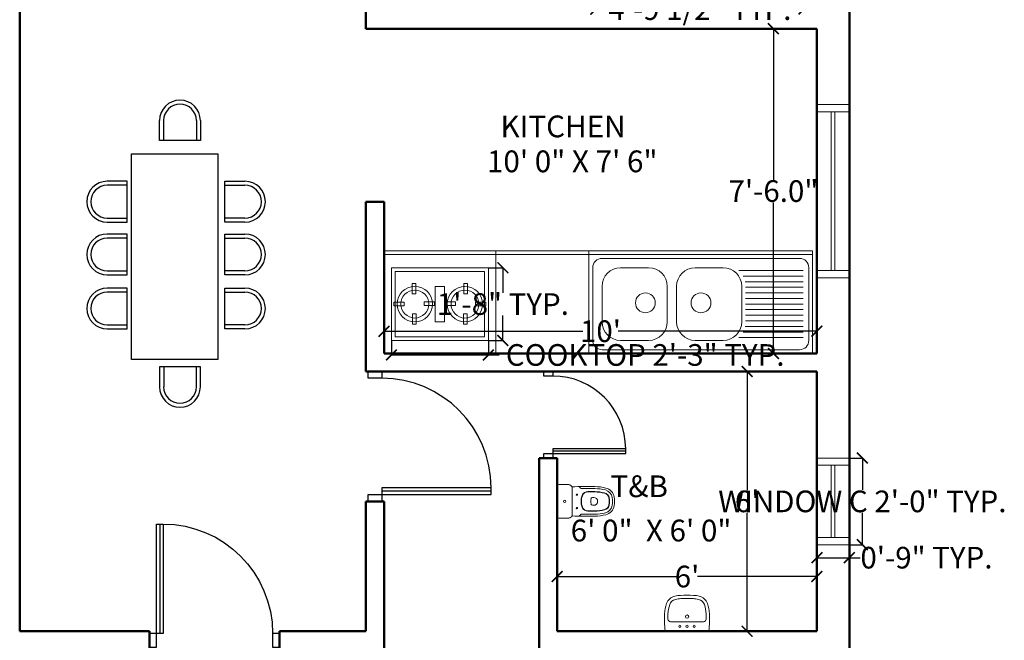
# Model space of a CAD drawing. Units: inches. Extents: x 147 to 1638, y 107 to 941.
# Tile 15 of 17: x 1365 to 1638, y 398 to 570. Entities that reach past the tile are written whole.
import ezdxf

# ---------------------------------------------------------------- set-up
doc = ezdxf.new("R2010")
doc.units = ezdxf.units.IN
doc.header["$MEASUREMENT"] = 0
for name, color, linetype, lineweight in [('A-ANNO-DIMS', 2, 'Continuous', 15), ('A-AREA-IDEN', 7, 'Continuous', 18), ('A-Door', 150, 'Continuous', 25), ('A-EQPM', 8, 'Continuous', 18), ('A-FLOR-CASE', 9, 'Continuous', 20), ('A-FLOR-FIXT', 9, 'Continuous', 18), ('furniture', 50, 'Continuous', 18), ('walls', 7, 'Continuous', 50), ('windows', 3, 'Continuous', 20)]:
    doc.layers.add(name, color=color, linetype=linetype, lineweight=lineweight)
for name, color, linetype in [('A-Glaz', 92, 'Continuous'), ('NT', 1, 'Continuous'), ('家', 40, 'Continuous')]:
    doc.layers.add(name, color=color, linetype=linetype)
doc.styles.get("Standard").update_dxf_attribs({"font": 'arial.ttf'})
doc.dimstyles.get("Standard").update_dxf_attribs({"dimtxt": 6, "dimasz": 3, "dimexe": 0.18, "dimexo": 0.0625, "dimgap": 0.09, "dimtad": 0, "dimtih": 1, "dimtoh": 1, "dimdec": 1, "dimzin": 0, "dimdsep": 46, "dimlunit": 3, "dimtxsty": 'Standard', "dimblk": 'ARCHTICK', "dimcen": 0.09, "dimadec": 0, "dimazin": 0, "dimtfac": 1, "dimtdec": 1, "dimtofl": 0, "dimtmove": 0, "dimatfit": 3, "dimfxl": 1, "dimtolj": 1, "dimtzin": 0, "dimarcsym": 0})

# ---------------------------------------------------------------- blocks, each defined once
blk = doc.blocks.new('A$C087A3AA9')
at = {"layer": 'A-Door'}
for points in [[(852.6, 94.7), (852.6, 852.6), (805.3, 852.6), (805.3, 94.7)], [(47.4, 94.7), (47.4, 0), (0, 0), (0, 94.7)], [(900, 94.7), (900, 0), (852.6, 0), (852.6, 94.7)]]:
    blk.add_lwpolyline(points, close=True, dxfattribs=at)
at = {"layer": 'A-Glaz'}
blk.add_line((828.9, 852.6), (828.9, 94.7), dxfattribs=at)
at = {"layer": 'NT'}
blk.add_arc((805.3, 94.7), 757.9, 90, 180, dxfattribs=at)
blk = doc.blocks.new('_ArchTick')
at = {"color": 0, "linetype": 'ByBlock', "const_width": 0.15}
blk.add_lwpolyline([(-0.5, -0.5), (0.5, 0.5)], dxfattribs=at)
blk = doc.blocks.new('*D40')
at = {"layer": 'A-ANNO-DIMS', "color": 0, "lineweight": -2, "transparency": 16777216}
for p, q in [((1566.2, 472.72), (1566.6, 472.72)), ((1566.42, 472.72), (1566.42, 439.87)), ((1566.42, 400.72), (1566.42, 433.56)), ((1566.2, 400.72), (1566.6, 400.72))]:
    blk.add_line(p, q, dxfattribs=at)
at = {"layer": 'Defpoints', "color": 0, "lineweight": -2, "transparency": 16777216}
for p in [(1566.14, 472.72), (1566.14, 400.72), (1566.42, 400.72)]:
    blk.add_point(p, dxfattribs=at)
at = {"layer": 'A-ANNO-DIMS', "color": 0, "lineweight": -2, "transparency": 16777216, "xscale": 3, "yscale": 3, "zscale": 3}
for p, rotation in [((1566.42, 472.72), 90), ((1566.42, 400.72), 270)]:
    blk.add_blockref('_ArchTick', p, dxfattribs=dict(at, rotation=rotation))
at = {"layer": 'A-ANNO-DIMS', "color": 0, "transparency": 16777216, "insert": (1566.42, 436.72), "char_height": 6, "attachment_point": 5}
blk.add_mtext("\\A1;6'", dxfattribs=at)
blk = doc.blocks.new('*D41')
at = {"layer": 'A-ANNO-DIMS', "color": 0, "lineweight": -2, "transparency": 16777216}
for p, q in [((1513.77, 415.95), (1513.77, 416.07)), ((1513.77, 415.89), (1546.9, 415.89)), ((1585.77, 415.89), (1552.63, 415.89)), ((1585.77, 415.95), (1585.77, 416.07))]:
    blk.add_line(p, q, dxfattribs=at)
at = {"layer": 'Defpoints', "color": 0, "lineweight": -2, "transparency": 16777216}
for p in [(1513.77, 415.89), (1585.77, 415.89), (1585.77, 415.89)]:
    blk.add_point(p, dxfattribs=at)
at = {"layer": 'A-ANNO-DIMS', "color": 0, "lineweight": -2, "transparency": 16777216, "xscale": 3, "yscale": 3, "zscale": 3, "rotation": 180}
blk.add_blockref('_ArchTick', (1513.77, 415.89), dxfattribs=at)
at = {"layer": 'A-ANNO-DIMS', "color": 0, "lineweight": -2, "transparency": 16777216, "xscale": 3, "yscale": 3, "zscale": 3}
blk.add_blockref('_ArchTick', (1585.77, 415.89), dxfattribs=at)
at = {"layer": 'A-ANNO-DIMS', "color": 0, "transparency": 16777216, "insert": (1549.77, 415.89), "char_height": 6, "attachment_point": 5}
blk.add_mtext("\\A1;6'", dxfattribs=at)
blk = doc.blocks.new('*D42')
at = {"layer": 'A-ANNO-DIMS', "color": 0, "lineweight": -2, "transparency": 16777216}
for p, q in [((1575.63, 567.72), (1573.54, 567.72)), ((1573.72, 567.72), (1573.72, 525.87)), ((1573.72, 477.72), (1573.72, 519.56)), ((1575.63, 477.72), (1573.54, 477.72))]:
    blk.add_line(p, q, dxfattribs=at)
at = {"layer": 'Defpoints', "color": 0, "lineweight": -2, "transparency": 16777216}
for p in [(1575.7, 567.72), (1573.72, 477.72), (1575.7, 477.72)]:
    blk.add_point(p, dxfattribs=at)
at = {"layer": 'A-ANNO-DIMS', "color": 0, "lineweight": -2, "transparency": 16777216, "xscale": 3, "yscale": 3, "zscale": 3}
for p, rotation in [((1573.72, 567.72), 90), ((1573.72, 477.72), 270)]:
    blk.add_blockref('_ArchTick', p, dxfattribs=dict(at, rotation=rotation))
at = {"layer": 'A-ANNO-DIMS', "color": 0, "transparency": 16777216, "insert": (1573.72, 522.72), "char_height": 6, "attachment_point": 5}
blk.add_mtext('\\A1;7\'-6.0"', dxfattribs=at)
blk = doc.blocks.new('*D43')
at = {"layer": 'A-ANNO-DIMS', "color": 0, "lineweight": -2, "transparency": 16777216}
for p, q in [((1465.77, 483.94), (1465.77, 484.06)), ((1465.77, 483.88), (1520.87, 483.88)), ((1585.77, 483.88), (1530.67, 483.88)), ((1585.77, 483.94), (1585.77, 484.06))]:
    blk.add_line(p, q, dxfattribs=at)
at = {"layer": 'Defpoints', "color": 0, "lineweight": -2, "transparency": 16777216}
for p in [(1465.77, 483.88), (1585.77, 483.88), (1585.77, 483.88)]:
    blk.add_point(p, dxfattribs=at)
at = {"layer": 'A-ANNO-DIMS', "color": 0, "lineweight": -2, "transparency": 16777216, "xscale": 3, "yscale": 3, "zscale": 3, "rotation": 180}
blk.add_blockref('_ArchTick', (1465.77, 483.88), dxfattribs=at)
at = {"layer": 'A-ANNO-DIMS', "color": 0, "lineweight": -2, "transparency": 16777216, "xscale": 3, "yscale": 3, "zscale": 3}
blk.add_blockref('_ArchTick', (1585.77, 483.88), dxfattribs=at)
at = {"layer": 'A-ANNO-DIMS', "color": 0, "transparency": 16777216, "insert": (1525.77, 483.88), "char_height": 6, "attachment_point": 5}
blk.add_mtext("\\A1;10'", dxfattribs=at)
blk = doc.blocks.new('2SAINDA')
at = {"color": 0, "linetype": 'ByBlock'}
for p, q in [((0, 0.188), (0, -0.188)), ((0.018, 0.2), (0.141, 0.2)), ((0.157, 0.192), (0.162, 0.188)), ((0.18, -0.164), (0.18, 0.164)), ((0.279, 0.159), (0.261, 0.176)), ((0.437, 0.047), (0.424, 0.047)), ((0.437, -0.047), (0.424, -0.047)), ((0.018, -0.2), (0.141, -0.2)), ((0.157, -0.192), (0.162, -0.188)), ((0.279, -0.159), (0.261, -0.176))]:
    blk.add_line(p, q, dxfattribs=at)
for centre, radius in [((0.09, 0), 0.0135), ((0.09, 0), 0.0135), ((0.236, 0.08), 0.0075), ((0.236, -0.08), 0.0075)]:
    blk.add_circle(centre, radius, dxfattribs=at)
for centre, radius, start, end in [((0.018, 0.18), 0.02, 90, 155.6901), ((0.141, 0.181), 0.019, 34.9372, 90), ((0.155, 0.164), 0.025, 23.3776, 73.7848), ((0.383, -5.322), 5.5, 89.2905, 92.1362), ((0.155, 0.164), 0.025, 360, 23.3776), ((0.293, 0.173), 0.02, 225, 270.9364), ((0.383, -5.322), 5.476, 89.2905, 90.9364), ((0.368, 0.043), 0.075, 90.1648, 160.016), ((0.383, -5.322), 5.44, 89.2905, 90.1648), ((0.444, -0.373), 0.55, 75.4605, 89.2905), ((0.444, -0.373), 0.526, 75.4605, 89.2905), ((0.549, 0.03), 0.11, 8.8162, 75.4605), ((0.549, 0.03), 0.134, 8.8162, 75.4605), ((0.485, 0), 0.2, 160.016, 199.984), ((0.485, 0), 0.196, 160.016, 199.984), ((0.368, 0.043), 0.071, 90.1648, 160.016), ((0.383, -5.322), 5.436, 89.2905, 90.1648), ((0.582, 0), 0.18, 170.2849, 189.7151), ((0.424, 0.027), 0.02, 90, 170.2849), ((0.437, 0), 0.047, 0, 90), ((0.437, 0), 0.047, 270, 0), ((0.444, -0.373), 0.49, 75.4605, 89.2905), ((0.444, -0.373), 0.486, 75.4605, 89.2905), ((0.549, 0.03), 0.07, 8.8162, 75.4605), ((0.549, 0.03), 0.074, 8.8162, 75.4605), ((0.355, 0), 0.266, 351.1838, 8.8162), ((0.355, 0), 0.27, 351.1838, 8.8162), ((0.355, 0), 0.306, 351.1838, 8.8162), ((0.355, 0), 0.33, 351.1838, 8.8162), ((0.368, -0.043), 0.075, 199.984, 269.8352), ((0.368, -0.043), 0.071, 199.984, 269.8352), ((0.383, 5.322), 5.436, 269.8352, 270.7095), ((0.383, 5.322), 5.44, 269.8352, 270.7095), ((0.424, -0.027), 0.02, 189.7151, 270), ((0.444, 0.373), 0.486, 270.7095, 284.5395), ((0.444, 0.373), 0.49, 270.7095, 284.5395), ((0.549, -0.03), 0.07, 284.5395, 351.1838), ((0.549, -0.03), 0.074, 284.5395, 351.1838), ((0.549, -0.03), 0.11, 284.5395, 351.1838), ((0.549, -0.03), 0.134, 284.5395, 351.1838), ((0.018, -0.18), 0.02, 204.3099, 270), ((0.141, -0.181), 0.019, 270, 325.0628), ((0.155, -0.164), 0.025, 286.2152, 336.6224), ((0.155, -0.164), 0.025, 336.6224, 0), ((0.383, 5.322), 5.5, 267.8638, 270.7095), ((0.293, -0.173), 0.02, 89.0636, 135), ((0.383, 5.322), 5.476, 269.0636, 270.7095), ((0.444, 0.373), 0.526, 270.7095, 284.5395), ((0.444, 0.373), 0.55, 270.7095, 284.5395)]:
    blk.add_arc(centre, radius, start, end, dxfattribs=at)
blk = doc.blocks.new('2SALADA2')
at = {"color": 0}
for p, q in [((-0.296, 0), (0.296, 0)), ((0.207, -0.13), (-0.207, -0.13))]:
    blk.add_line(p, q, dxfattribs=at)
for centre, radius in [((-0.1, -0.07), 0.015), ((0, -0.07), 0.0175), ((0.1, -0.07), 0.015), ((0, -0.205), 0.023)]:
    blk.add_circle(centre, radius, dxfattribs=at)
for centre, radius, start, end in [((-0.296, -0.01), 0.01, 90, 173.6262), ((0.296, -0.01), 0.01, 6.3738, 90), ((1.185, -0.175), 1.5, 173.6262, 182.693), ((-0.227, -0.171), 0.04, 95.5937, 179.6995), ((-0.207, -0.38), 0.25, 90, 95.5937), ((0.207, -0.38), 0.25, 84.4063, 90), ((0.227, -0.171), 0.04, 0.3005, 84.4063), ((-1.185, -0.175), 1.5, 357.307, 6.3738), ((0.186, -0.222), 0.5, 182.693, 199.3406), ((1.186, -0.221), 1.454, 178.0234, 180.898), ((0.186, -0.222), 0.454, 182.693, 199.3406), ((-0.186, -0.222), 0.454, 340.6594, 357.307), ((-1.186, -0.221), 1.454, 359.102, 1.9766), ((-0.186, -0.222), 0.5, 340.6594, 357.307), ((-0.135, -0.335), 0.16, 199.3406, 257.4429), ((-0.135, -0.335), 0.114, 199.3406, 257.4429), ((0.135, -0.335), 0.114, 282.5571, 340.6594), ((0.135, -0.335), 0.16, 282.5571, 340.6594), ((-0.061, -0.003), 0.5, 257.4429, 266.4982), ((-0.061, -0.003), 0.454, 257.4429, 266.4982), ((0, 0.995), 1.5, 266.4982, 273.5018), ((0, 0.995), 1.454, 266.4982, 273.5018), ((0.061, -0.003), 0.454, 273.5018, 282.5571), ((0.061, -0.003), 0.5, 273.5018, 282.5571)]:
    blk.add_arc(centre, radius, start, end, dxfattribs=at)
blk = doc.blocks.new('A$C45A766E2')
at = {"layer": '家'}
for p, q in [((0.363, 1.317), (0.363, 1.078)), ((0.412, 1.317), (0.412, 1.078)), ((0.801, 1.078), (0.801, 1.317)), ((0.849, 1.078), (0.849, 1.317)), ((1.006, 1.317), (1.006, 1.078)), ((1.054, 1.317), (1.054, 1.078)), ((1.443, 1.078), (1.443, 1.317)), ((1.492, 1.078), (1.492, 1.317)), ((1.634, 1.317), (1.634, 1.078)), ((1.683, 1.317), (1.683, 1.078)), ((2.072, 1.078), (2.072, 1.317)), ((2.12, 1.078), (2.12, 1.317)), ((0.363, 1.078), (0.849, 1.078)), ((0.363, 1.078), (0.849, 1.078)), ((1.006, 1.078), (1.492, 1.078)), ((1.006, 1.078), (1.492, 1.078)), ((1.634, 1.078), (2.12, 1.078)), ((1.634, 1.078), (2.12, 1.078)), ((0, 1.028), (2.445, 1.028)), ((0, 0), (0, 1.028)), ((2.445, 1.028), (2.445, 0)), ((-0.088, 0.693), (-0.327, 0.693)), ((-0.088, 0.644), (-0.327, 0.644)), ((-0.088, 0.207), (-0.088, 0.693)), ((-0.088, 0.207), (-0.088, 0.693)), ((2.604, 0.693), (2.843, 0.693)), ((2.604, 0.207), (2.604, 0.693)), ((2.604, 0.207), (2.604, 0.693)), ((2.604, 0.644), (2.843, 0.644)), ((-0.327, 0.255), (-0.088, 0.255)), ((2.843, 0.255), (2.604, 0.255)), ((-0.327, 0.207), (-0.088, 0.207)), ((2.843, 0.207), (2.604, 0.207)), ((2.445, 0), (0, 0)), ((0.363, -0.085), (0.849, -0.085)), ((0.363, -0.085), (0.849, -0.085)), ((0.363, -0.324), (0.363, -0.085)), ((0.412, -0.324), (0.412, -0.085)), ((0.801, -0.085), (0.801, -0.324)), ((0.849, -0.085), (0.849, -0.324)), ((1.006, -0.324), (1.006, -0.085)), ((1.006, -0.085), (1.492, -0.085)), ((1.006, -0.085), (1.492, -0.085)), ((1.054, -0.324), (1.054, -0.085)), ((1.443, -0.085), (1.443, -0.324)), ((1.492, -0.085), (1.492, -0.324)), ((1.634, -0.085), (2.12, -0.085)), ((1.634, -0.085), (2.12, -0.085)), ((1.634, -0.324), (1.634, -0.085)), ((1.683, -0.324), (1.683, -0.085)), ((2.072, -0.085), (2.072, -0.324)), ((2.12, -0.085), (2.12, -0.324))]:
    blk.add_line(p, q, dxfattribs=at)
for centre, radius, start, end in [((0.606, 1.317), 0.243, 0, 180), ((1.249, 1.317), 0.243, 0, 180), ((1.877, 1.317), 0.243, 0, 180), ((0.606, 1.317), 0.195, 0, 180), ((1.249, 1.317), 0.195, 0, 180), ((1.877, 1.317), 0.195, 0, 180), ((-0.327, 0.45), 0.243, 90, 270), ((-0.327, 0.45), 0.195, 90, 270), ((2.843, 0.45), 0.243, 270, 90), ((2.843, 0.45), 0.195, 270, 90), ((0.606, -0.324), 0.243, 180, 0), ((0.606, -0.324), 0.195, 180, 0), ((1.249, -0.324), 0.243, 180, 0), ((1.249, -0.324), 0.195, 180, 0), ((1.877, -0.324), 0.243, 180, 0), ((1.877, -0.324), 0.195, 180, 0)]:
    blk.add_arc(centre, radius, start, end, dxfattribs=at)
blk = doc.blocks.new('WIN-48IN')
for p, q in [((9, 48), (0, 48)), ((0, 48), (0, 0)), ((9, 0), (9, 48)), ((9, 46), (0, 46)), ((4, 2), (4, 46)), ((5, 2), (5, 46)), ((0, 2), (9, 2)), ((0, 0), (9, 0))]:
    blk.add_line(p, q)
blk = doc.blocks.new('WIN-24IN')
for p, q in [((9, 24), (0, 24)), ((0, 24), (0, 0)), ((9, 22), (0, 22)), ((4, 2), (4, 22)), ((5, 2), (5, 22)), ((9, 0), (9, 24)), ((0, 2), (9, 2)), ((0, 0), (9, 0))]:
    blk.add_line(p, q)
blk = doc.blocks.new('CABINET-KITCHEN-RUN')
for p, q in [((0, 28.41), (118.8, 28.41)), ((0, 0), (0, 28.41)), ((0, 27.38), (118.8, 27.38)), ((30.99, 0), (30.99, 28.41)), ((56.82, 0), (56.82, 28.41)), ((118.8, 28.41), (118.8, 0)), ((118.8, 0), (0, 0))]:
    blk.add_line(p, q)
blk = doc.blocks.new('COOKTOP-2-BURNER')
for p, q in [((0, 0), (0, 20.15)), ((0, 20.15), (26.86, 20.15)), ((1.03, 1.03), (1.03, 19.11)), ((1.03, 19.11), (25.83, 19.11)), ((25.83, 1.03), (25.83, 19.11)), ((26.86, 0), (26.86, 20.15)), ((5.75, 15.75), (5.75, 12.91)), ((5.75, 15.75), (6.79, 15.75)), ((6.79, 15.75), (6.79, 12.91)), ((12.14, 14.98), (14.72, 14.98)), ((12.14, 14.98), (12.14, 5.17)), ((14.72, 14.98), (14.72, 5.17)), ((21.11, 15.75), (20.07, 15.75)), ((20.07, 15.75), (20.07, 12.91)), ((21.11, 15.75), (21.11, 12.91)), ((5.75, 12.91), (6.79, 12.91)), ((21.11, 12.91), (20.07, 12.91)), ((0.69, 9.55), (0.69, 10.59)), ((0.69, 10.59), (3.53, 10.59)), ((0.69, 9.55), (3.53, 9.55)), ((3.53, 9.55), (3.53, 10.59)), ((11.95, 10.69), (9.11, 10.69)), ((9.11, 10.69), (9.11, 9.66)), ((11.95, 9.66), (9.11, 9.66)), ((11.95, 10.69), (11.95, 9.66)), ((14.91, 10.69), (17.75, 10.69)), ((14.91, 10.69), (14.91, 9.66)), ((14.91, 9.66), (17.75, 9.66)), ((17.75, 10.69), (17.75, 9.66)), ((23.33, 9.55), (23.33, 10.59)), ((26.17, 10.59), (23.33, 10.59)), ((26.17, 9.55), (23.33, 9.55)), ((26.17, 9.55), (26.17, 10.59)), ((5.86, 4.49), (5.86, 7.33)), ((6.89, 7.33), (5.86, 7.33)), ((6.89, 4.49), (6.89, 7.33)), ((19.97, 4.49), (19.97, 7.33)), ((19.97, 7.33), (21, 7.33)), ((21, 4.49), (21, 7.33)), ((6.89, 4.49), (5.86, 4.49)), ((12.14, 5.17), (14.72, 5.17)), ((19.97, 4.49), (21, 4.49)), ((0, 0), (26.86, 0)), ((1.03, 1.03), (25.83, 1.03))]:
    blk.add_line(p, q)
for centre, radius in [((6.48, 10.08), 4.91), ((6.48, 10.08), 3.87), ((20.38, 10.08), 4.91), ((20.38, 10.08), 3.87)]:
    blk.add_circle(centre, radius)
blk = doc.blocks.new('SINK-DOUBLE-DRAINBOARD')
for p, q in [((57.34, 25.31), (2.58, 25.31)), ((0, 22.73), (0, 2.58)), ((15.5, 22.73), (7.75, 22.73)), ((36.16, 22.73), (28.41, 22.73)), ((40.53, 21.95), (58.37, 21.95)), ((59.92, 2.58), (59.92, 22.73)), ((41.67, 20.4), (58.37, 20.4)), ((2.58, 17.56), (2.58, 7.75)), ((20.66, 17.56), (20.66, 7.75)), ((23.24, 17.56), (23.24, 7.75)), ((41.32, 17.56), (41.32, 7.75)), ((42.22, 18.85), (58.37, 18.85)), ((42.36, 17.3), (58.37, 17.3)), ((42.36, 15.75), (58.37, 15.75)), ((42.36, 14.2), (58.37, 14.2)), ((42.36, 12.66), (58.37, 12.66)), ((42.36, 11.11), (58.37, 11.11)), ((42.36, 9.56), (58.37, 9.56)), ((42.22, 6.46), (58.37, 6.46)), ((42.36, 8.01), (58.37, 8.01)), ((40.53, 3.36), (58.37, 3.36)), ((41.67, 4.91), (58.37, 4.91)), ((2.58, 0), (57.34, 0)), ((7.75, 2.58), (15.5, 2.58)), ((28.41, 2.58), (36.16, 2.58))]:
    blk.add_line(p, q)
for centre in [(14.61, 13), (30.02, 13)]:
    blk.add_circle(centre, 2.75)
for centre, radius, start, end in [((2.58, 22.73), 2.58, 90, 180), ((57.34, 22.73), 2.58, 0, 90), ((7.75, 17.56), 5.17, 90, 180), ((15.5, 17.56), 5.17, 0, 90), ((28.41, 17.56), 5.17, 90, 180), ((36.16, 17.56), 5.17, 0, 90), ((7.75, 7.75), 5.17, 180, 270), ((15.5, 7.75), 5.17, 270, 0), ((28.41, 7.75), 5.17, 180, 270), ((36.16, 7.75), 5.17, 270, 0), ((2.58, 2.58), 2.58, 180, 270), ((57.34, 2.58), 2.58, 270, 0)]:
    blk.add_arc(centre, radius, start, end)
blk = doc.blocks.new('*D106')
at = {"layer": 'A-ANNO-DIMS', "color": 0, "lineweight": -2, "transparency": 16777216}
for p, q in [((1594.83, 448.72), (1598.55, 448.72)), ((1598.37, 448.72), (1598.37, 439.91)), ((1598.37, 424.72), (1598.37, 433.52)), ((1594.83, 424.72), (1598.55, 424.72))]:
    blk.add_line(p, q, dxfattribs=at)
at = {"layer": 'Defpoints', "color": 0, "lineweight": -2, "transparency": 16777216}
for p in [(1594.77, 448.72), (1598.37, 448.72), (1594.77, 424.72)]:
    blk.add_point(p, dxfattribs=at)
at = {"layer": 'A-ANNO-DIMS', "color": 0, "lineweight": -2, "transparency": 16777216, "xscale": 3, "yscale": 3, "zscale": 3}
for p, rotation in [((1598.37, 448.72), 90), ((1598.37, 424.72), 270)]:
    blk.add_blockref('_ArchTick', p, dxfattribs=dict(at, rotation=rotation))
at = {"layer": 'A-ANNO-DIMS', "color": 0, "transparency": 16777216, "insert": (1598.37, 436.72), "char_height": 6, "attachment_point": 5}
blk.add_mtext('\\A1;WINDOW C 2\'-0" TYP.', dxfattribs=at)
blk = doc.blocks.new('*D107')
at = {"layer": 'A-ANNO-DIMS', "color": 0, "lineweight": -2, "transparency": 16777216}
for p, q in [((1585.77, 424.66), (1585.77, 420.94)), ((1594.77, 424.66), (1594.77, 420.94)), ((1585.77, 421.12), (1594.77, 421.12)), ((1594.77, 421.12), (1597.77, 421.12))]:
    blk.add_line(p, q, dxfattribs=at)
at = {"layer": 'Defpoints', "color": 0, "lineweight": -2, "transparency": 16777216}
for p in [(1585.77, 424.72), (1594.77, 424.72), (1594.77, 421.12)]:
    blk.add_point(p, dxfattribs=at)
at = {"layer": 'A-ANNO-DIMS', "color": 0, "lineweight": -2, "transparency": 16777216, "xscale": 3, "yscale": 3, "zscale": 3, "rotation": 180}
blk.add_blockref('_ArchTick', (1585.77, 421.12), dxfattribs=at)
at = {"layer": 'A-ANNO-DIMS', "color": 0, "lineweight": -2, "transparency": 16777216, "xscale": 3, "yscale": 3, "zscale": 3}
blk.add_blockref('_ArchTick', (1594.77, 421.12), dxfattribs=at)
at = {"layer": 'A-ANNO-DIMS', "color": 0, "transparency": 16777216, "insert": (1616.14, 421.12), "char_height": 6, "attachment_point": 5}
blk.add_mtext('\\A1;0\'-9" TYP.', dxfattribs=at)
blk = doc.blocks.new('*D113')
at = {"layer": 'A-ANNO-DIMS', "color": 0, "lineweight": -2, "transparency": 16777216}
for p, q in [((1524.46, 583.32), (1524.46, 572.97)), ((1582.2, 583.32), (1582.2, 572.97)), ((1524.46, 573.15), (1527.84, 573.15)), ((1582.2, 573.15), (1578.82, 573.15))]:
    blk.add_line(p, q, dxfattribs=at)
at = {"layer": 'Defpoints', "color": 0, "lineweight": -2, "transparency": 16777216}
for p in [(1524.46, 583.38), (1582.2, 583.38), (1524.46, 573.15)]:
    blk.add_point(p, dxfattribs=at)
at = {"layer": 'A-ANNO-DIMS', "color": 0, "lineweight": -2, "transparency": 16777216, "xscale": 3, "yscale": 3, "zscale": 3, "rotation": 180}
blk.add_blockref('_ArchTick', (1524.46, 573.15), dxfattribs=at)
at = {"layer": 'A-ANNO-DIMS', "color": 0, "lineweight": -2, "transparency": 16777216, "xscale": 3, "yscale": 3, "zscale": 3}
blk.add_blockref('_ArchTick', (1582.2, 573.15), dxfattribs=at)
at = {"layer": 'A-ANNO-DIMS', "color": 0, "transparency": 16777216, "insert": (1553.33, 573.15), "char_height": 6, "attachment_point": 5}
blk.add_mtext('\\A1;4\'-9 1/2" TYP.', dxfattribs=at)
blk = doc.blocks.new('*D124')
at = {"layer": 'A-ANNO-DIMS', "color": 0, "lineweight": -2, "transparency": 16777216}
for p, q in [((1467.83, 481.27), (1467.83, 477.12)), ((1494.69, 481.27), (1494.69, 477.12)), ((1467.83, 477.3), (1494.69, 477.3)), ((1494.69, 477.3), (1497.69, 477.3))]:
    blk.add_line(p, q, dxfattribs=at)
at = {"layer": 'Defpoints', "color": 0, "lineweight": -2, "transparency": 16777216}
for p in [(1467.83, 481.33), (1494.69, 481.33), (1494.69, 477.3)]:
    blk.add_point(p, dxfattribs=at)
at = {"layer": 'A-ANNO-DIMS', "color": 0, "lineweight": -2, "transparency": 16777216, "xscale": 3, "yscale": 3, "zscale": 3, "rotation": 180}
blk.add_blockref('_ArchTick', (1467.83, 477.3), dxfattribs=at)
at = {"layer": 'A-ANNO-DIMS', "color": 0, "lineweight": -2, "transparency": 16777216, "xscale": 3, "yscale": 3, "zscale": 3}
blk.add_blockref('_ArchTick', (1494.69, 477.3), dxfattribs=at)
at = {"layer": 'A-ANNO-DIMS', "color": 0, "transparency": 16777216, "insert": (1538.16, 477.3), "char_height": 6, "attachment_point": 5}
blk.add_mtext('\\A1;COOKTOP 2\'-3" TYP.', dxfattribs=at)
blk = doc.blocks.new('*D125')
at = {"layer": 'A-ANNO-DIMS', "color": 0, "lineweight": -2, "transparency": 16777216}
for p, q in [((1494.76, 501.48), (1498.9, 501.48)), ((1498.72, 501.48), (1498.72, 494.56)), ((1498.72, 481.33), (1498.72, 488.25)), ((1494.76, 481.33), (1498.9, 481.33))]:
    blk.add_line(p, q, dxfattribs=at)
at = {"layer": 'Defpoints', "color": 0, "lineweight": -2, "transparency": 16777216}
for p in [(1494.69, 501.48), (1498.72, 501.48), (1494.69, 481.33)]:
    blk.add_point(p, dxfattribs=at)
at = {"layer": 'A-ANNO-DIMS', "color": 0, "lineweight": -2, "transparency": 16777216, "xscale": 3, "yscale": 3, "zscale": 3}
for p, rotation in [((1498.72, 501.48), 90), ((1498.72, 481.33), 270)]:
    blk.add_blockref('_ArchTick', p, dxfattribs=dict(at, rotation=rotation))
at = {"layer": 'A-ANNO-DIMS', "color": 0, "transparency": 16777216, "insert": (1498.72, 491.41), "char_height": 6, "attachment_point": 5}
blk.add_mtext('\\A1;1\'-8" TYP.', dxfattribs=at)

msp = doc.modelspace()

# ---------------------------------------------------------------- linework, layer by layer
at = {"layer": 'walls'}
for p, q in [((1594.77, 909.72), (1594.77, 201.72)), ((1364.77, 722.72), (1364.77, 400.72)), ((1460.77, 572.72), (1460.77, 567.72)), ((1465.77, 567.72), (1460.77, 567.72)), ((1465.77, 567.72), (1585.77, 567.72)), ((1585.77, 567.72), (1585.77, 477.72)), ((1460.77, 519.72), (1460.77, 472.72)), ((1465.77, 519.72), (1460.77, 519.72)), ((1465.77, 519.72), (1465.77, 477.72)), ((1465.77, 477.72), (1585.77, 477.72)), ((1465.77, 472.72), (1460.77, 472.72)), ((1465.77, 472.72), (1508.77, 472.72)), ((1508.77, 472.72), (1513.77, 472.72)), ((1513.77, 472.72), (1585.77, 472.72)), ((1585.77, 472.72), (1585.77, 400.72)), ((1508.77, 448.72), (1508.77, 395.72)), ((1508.77, 448.72), (1513.77, 448.72)), ((1513.77, 448.72), (1513.77, 400.72)), ((1460.77, 436.72), (1460.77, 400.72)), ((1465.77, 436.72), (1460.77, 436.72)), ((1465.77, 436.72), (1465.77, 210.72)), ((1364.77, 400.72), (1388.77, 400.72)), ((1388.77, 400.72), (1400.77, 400.72)), ((1400.77, 400.72), (1400.77, 395.72)), ((1436.77, 400.72), (1460.77, 400.72)), ((1436.77, 400.72), (1436.77, 395.72)), ((1513.77, 400.72), (1585.77, 400.72))]:
    msp.add_line(p, q, dxfattribs=at)

# ---------------------------------------------------------------- block references
at = {"layer": 'A-Door', "rotation": 270}
for p, xscale, yscale, zscale in [((1461.37, 472.72), 0.0400000000000001, 0.0400000000000001, 0.0400000000000001), ((1510.03, 472.72), 0.0266666667542921, 0.0266666667542921, 0.0266666667542921)]:
    msp.add_blockref('A$C087A3AA9', p, dxfattribs=dict(at, xscale=xscale, yscale=yscale, zscale=zscale))
at = {"layer": 'A-Door', "xscale": -0.0400000000000001, "yscale": 0.0400000000000001, "zscale": 0.0400000000000001}
msp.add_blockref('A$C087A3AA9', (1436.77, 396.32), dxfattribs=at)
at = {"layer": 'A-EQPM'}
msp.add_blockref('COOKTOP-2-BURNER', (1467.83, 481.33), dxfattribs=at)
at = {"layer": 'A-FLOR-CASE'}
msp.add_blockref('CABINET-KITCHEN-RUN', (1465.77, 477.72), dxfattribs=at)
at = {"layer": 'A-FLOR-FIXT'}
msp.add_blockref('SINK-DOUBLE-DRAINBOARD', (1523.62, 478.75), dxfattribs=at)
at = {"layer": 'A-FLOR-FIXT', "xscale": 23.19012112898009, "yscale": 23.19012112898009, "zscale": 23.19012112898009}
msp.add_blockref('2SAINDA', (1513.77, 436.72), dxfattribs=at)
at = {"layer": 'A-FLOR-FIXT', "xscale": 19.81841434140962, "yscale": 19.81841434140962, "zscale": 19.81841434140962, "rotation": 180}
msp.add_blockref('2SALADA2', (1549.77, 400.72), dxfattribs=at)
at = {"layer": 'furniture', "xscale": 23.28367368005433, "yscale": 23.28367368005433, "zscale": 23.28367368005433, "rotation": 90}
msp.add_blockref('A$C45A766E2', (1419.68, 476.07), dxfattribs=at)
at = {"layer": 'windows'}
for name, p in [('WIN-48IN', (1585.77, 498.72)), ('WIN-24IN', (1585.77, 424.72))]:
    msp.add_blockref(name, p, dxfattribs=at)

# ---------------------------------------------------------------- texts
at = {"layer": 'A-AREA-IDEN'}
for s, height, p in [('KITCHEN ', 6.031, (1498.05, 537.63)), ('  10\' 0" X 7\' 6"', 6.0306, (1490.61, 527.94)), ('T&B', 6.031, (1528.55, 437.89)), ('  6\' 0"  X 6\' 0"', 6.0306, (1513.83, 425.62))]:
    msp.add_text(s, height=height, dxfattribs=at).set_placement(p)

# ---------------------------------------------------------------- dimensions: what is measured, and where the dimension line sits
at = {"layer": 'A-ANNO-DIMS'}
for base, p1, p2, angle, text, picture, middle in [((1524.46, 573.15), (1582.2, 583.38), (1524.46, 583.38), 180, '<> TYP.', '*D113', (1553.33, 573.15)), ((1498.7231, 501.4788), (1494.6941, 481.3337), (1494.6941, 501.4788), 90, '<> TYP.', '*D125', (1498.7231, 491.4062)), ((1598.37, 448.72), (1594.77, 424.72), (1594.77, 448.72), 90, 'WINDOW C <> TYP.', '*D106', (1598.37, 436.72))]:
    dim = msp.add_linear_dim(base=base, p1=p1, p2=p2, angle=angle, text=text, dimstyle='Standard', override={"dimdec": 1, "dimlfac": 1, "dimrnd": 0, "dimzin": 1, "dimdsep": 46, "dimlunit": 4, "dimfrac": 2}, dxfattribs=at)
    dim.commit()
    dim.dimension.update_dxf_attribs({"geometry": picture, "text_midpoint": middle})
for base, p1, p2, picture, middle in [((1573.72, 477.72), (1575.7, 567.72), (1575.7, 477.72), '*D42', (1573.72, 522.72)), ((1566.42, 400.72), (1566.14, 472.72), (1566.14, 400.72), '*D40', (1566.42, 436.72))]:
    dim = msp.add_linear_dim(base=base, p1=p1, p2=p2, angle=90, dimstyle='Standard', override={"dimclrd": 0, "dimclre": 0, "dimclrt": 0}, dxfattribs=at)
    dim.commit()
    dim.dimension.update_dxf_attribs({"geometry": picture, "text_midpoint": middle})
for base, p1, p2, text, picture, middle in [((1494.69, 477.3), (1467.83, 481.33), (1494.69, 481.33), 'COOKTOP <> TYP.', '*D124', (1538.16, 477.3)), ((1594.77, 421.12), (1585.77, 424.72), (1594.77, 424.72), '<> TYP.', '*D107', (1616.14, 421.12))]:
    dim = msp.add_linear_dim(base=base, p1=p1, p2=p2, text=text, dimstyle='Standard', override={"dimdec": 1, "dimlfac": 1, "dimrnd": 0, "dimzin": 1, "dimdsep": 46, "dimlunit": 4, "dimfrac": 2}, dxfattribs=at)
    dim.commit()
    dim.dimension.update_dxf_attribs({"geometry": picture, "text_midpoint": middle})
for base, p1, p2, picture, middle in [((1585.77, 483.88), (1465.77, 483.88), (1585.77, 483.88), '*D43', (1525.77, 483.88)), ((1585.77, 415.89), (1513.77, 415.89), (1585.77, 415.89), '*D41', (1549.77, 415.89))]:
    dim = msp.add_linear_dim(base=base, p1=p1, p2=p2, dimstyle='Standard', override={"dimclrd": 0, "dimclre": 0, "dimclrt": 0}, dxfattribs=at)
    dim.commit()
    dim.dimension.update_dxf_attribs({"geometry": picture, "text_midpoint": middle})

doc.saveas('drawing.dxf')
